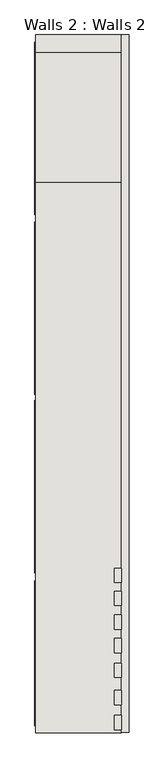
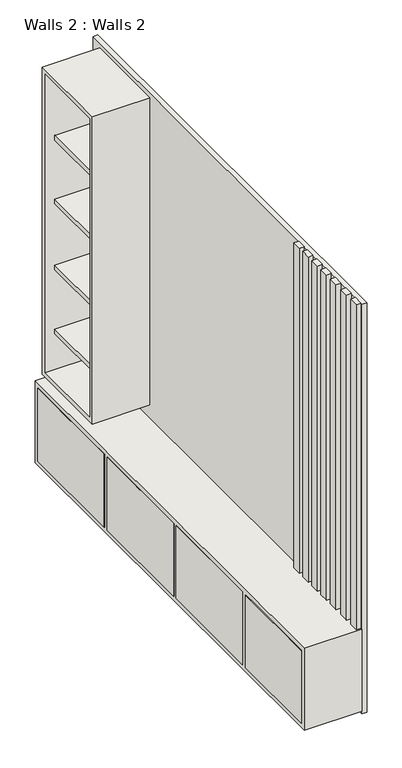
"""IFC4 building model written with IfcOpenShell, lengths in millimetres: wall geometry, Walls 2 : Walls 2."""

from ifc_helpers import new_model, si_unit, frame, origin, origin_with_axes, place, context, project, spatial, polyline, outline, extrude, faceted_brep, source, transform, mapped, element, save


def walls_2_walls_2_a3e54821(model_context):
    return source(origin(), model_context, "Body", "SolidModel", [
        extrude(outline(polyline([(-1167.1478577, -3563.611411), (-1167.1478577, -3052.3039411), (-1164.5681702, -3052.3039411), (-1164.5681702, -3563.611411), (-1167.1478577, -3563.611411)])), frame((0.0, 0.0, 40.132709), z_axis=(0.0, 0.0, 1.0), x_axis=(1.0, 0.0, 0.0)), (0.0, 0.0, 1.0), 406.4),
        extrude(outline(polyline([(-1167.1478577, -3023.861411), (-1167.1478577, -2414.261411), (-1164.5681702, -2414.261411), (-1164.5681702, -3023.861411), (-1167.1478577, -3023.861411)])), frame((0.0, 0.0, 40.132709), z_axis=(0.0, 0.0, 1.0), x_axis=(1.0, 0.0, 0.0)), (0.0, 0.0, 1.0), 406.4),
        extrude(outline(polyline([(-1167.1478577, -2393.557676), (-1167.1478577, -1783.957676), (-1164.5681702, -1783.957676), (-1164.5681702, -2393.557676), (-1167.1478577, -2393.557676)])), frame((0.0, 0.0, 40.132709), z_axis=(0.0, 0.0, 1.0), x_axis=(1.0, 0.0, 0.0)), (0.0, 0.0, 1.0), 406.4),
        extrude(outline(polyline([(-1167.1478577, -1758.557676), (-1167.1478577, -1148.957676), (-1164.5681702, -1148.957676), (-1164.5681702, -1758.557676), (-1167.1478577, -1758.557676)])), frame((0.0, 0.0, 40.132709), z_axis=(0.0, 0.0, 1.0), x_axis=(1.0, 0.0, 0.0)), (0.0, 0.0, 1.0), 406.4),
        extrude(outline(polyline([(-885.1681702, -3577.3260888), (-885.1681702, -3526.5260888), (-859.7681702, -3526.5260888), (-859.7681702, -3577.3260888), (-885.1681702, -3577.3260888)])), frame((0.0, 0.0, 471.932709), z_axis=(0.0, 0.0, 1.0), x_axis=(1.0, 0.0, 0.0)), (0.0, 0.0, 1.0), 1815.6625633),
        extrude(outline(polyline([(-885.1681702, -3489.4392633), (-885.1681702, -3438.6392633), (-859.7681702, -3438.6392633), (-859.7681702, -3489.4392633), (-885.1681702, -3489.4392633)])), frame((0.0, 0.0, 471.932709), z_axis=(0.0, 0.0, 1.0), x_axis=(1.0, 0.0, 0.0)), (0.0, 0.0, 1.0), 1815.6625633),
        extrude(outline(polyline([(-885.1681702, -3222.7392633), (-885.1681702, -3171.9392633), (-859.7681702, -3171.9392633), (-859.7681702, -3222.7392633), (-885.1681702, -3222.7392633)])), frame((0.0, 0.0, 471.932709), z_axis=(0.0, 0.0, 1.0), x_axis=(1.0, 0.0, 0.0)), (0.0, 0.0, 1.0), 1815.6625633),
        extrude(outline(polyline([(-885.1681702, -3393.1760888), (-885.1681702, -3342.3760888), (-859.7681702, -3342.3760888), (-859.7681702, -3393.1760888), (-885.1681702, -3393.1760888)])), frame((0.0, 0.0, 471.932709), z_axis=(0.0, 0.0, 1.0), x_axis=(1.0, 0.0, 0.0)), (0.0, 0.0, 1.0), 1815.6625633),
        extrude(outline(polyline([(-885.1681702, -3305.2892633), (-885.1681702, -3254.4892633), (-859.7681702, -3254.4892633), (-859.7681702, -3305.2892633), (-885.1681702, -3305.2892633)])), frame((0.0, 0.0, 471.932709), z_axis=(0.0, 0.0, 1.0), x_axis=(1.0, 0.0, 0.0)), (0.0, 0.0, 1.0), 1815.6625633),
        extrude(outline(polyline([(-885.1681702, -3139.1760888), (-885.1681702, -3088.3760888), (-859.7681702, -3088.3760888), (-859.7681702, -3139.1760888), (-885.1681702, -3139.1760888)])), frame((0.0, 0.0, 471.932709), z_axis=(0.0, 0.0, 1.0), x_axis=(1.0, 0.0, 0.0)), (0.0, 0.0, 1.0), 1815.6625633),
        extrude(outline(polyline([(-885.1681702, -3057.9595435), (-885.1681702, -3007.1595435), (-859.7681702, -3007.1595435), (-859.7681702, -3057.9595435), (-885.1681702, -3057.9595435)])), frame((0.0, 0.0, 471.932709), z_axis=(0.0, 0.0, 1.0), x_axis=(1.0, 0.0, 0.0)), (0.0, 0.0, 1.0), 1815.6625633),
        extrude(outline(polyline([(-1164.5681702, -3587.357676), (-1164.5681702, -1123.557676), (-859.7681702, -1123.557676), (-859.7681702, -3587.357676), (-1164.5681702, -3587.357676)])), frame((0.0, 0.0, 14.732709), z_axis=(0.0, 0.0, 1.0), x_axis=(1.0, 0.0, 0.0)), (0.0, 0.0, 1.0), 457.2),
        extrude(outline(polyline([(-1113.7681702, -1618.857676), (-1113.7681702, -1212.457676), (-885.1681702, -1212.457676), (-885.1681702, -1618.857676), (-1113.7681702, -1618.857676)])), frame((0.0, 0.0, 1852.4679591), z_axis=(0.0, 0.0, 1.0), x_axis=(1.0, 0.0, 0.0)), (0.0, 0.0, 1.0), 25.4),
        extrude(outline(polyline([(-1113.7681702, -1618.857676), (-1113.7681702, -1212.457676), (-885.1681702, -1212.457676), (-885.1681702, -1618.857676), (-1113.7681702, -1618.857676)])), frame((0.0, 0.0, 1496.8679591), z_axis=(0.0, 0.0, 1.0), x_axis=(1.0, 0.0, 0.0)), (0.0, 0.0, 1.0), 25.4),
        extrude(outline(polyline([(-1113.7681702, -1618.857676), (-1113.7681702, -1212.457676), (-885.1681702, -1212.457676), (-885.1681702, -1618.857676), (-1113.7681702, -1618.857676)])), frame((0.0, 0.0, 1128.5679591), z_axis=(0.0, 0.0, 1.0), x_axis=(1.0, 0.0, 0.0)), (0.0, 0.0, 1.0), 25.4),
        extrude(outline(polyline([(-1113.7681702, -1618.857676), (-1113.7681702, -1212.457676), (-885.1681702, -1212.457676), (-885.1681702, -1618.857676), (-1113.7681702, -1618.857676)])), frame((0.0, 0.0, 771.5696931), z_axis=(0.0, 0.0, 1.0), x_axis=(1.0, 0.0, 0.0)), (0.0, 0.0, 1.0), 25.4),
        faceted_brep([(-1164.5681702, -1644.257676, 2262.1952722), (-1164.5681702, -1187.057676, 2262.1952722), (-1164.5681702, -1187.057676, 545.99238), (-1164.5681702, -1644.257676, 545.99238), (-1164.5681702, -1618.857676, 2236.7952722), (-1164.5681702, -1618.857676, 571.39238), (-1164.5681702, -1212.457676, 571.39238), (-1164.5681702, -1212.457676, 2236.7952722), (-859.7681702, -1644.257676, 2262.1952722), (-859.7681702, -1644.257676, 545.99238), (-859.7681702, -1187.057676, 545.99238), (-859.7681702, -1187.057676, 2262.1952722), (-885.1681702, -1618.857676, 2236.7952722), (-885.1681702, -1212.457676, 2236.7952722), (-885.1681702, -1212.457676, 571.39238), (-885.1681702, -1618.857676, 571.39238)], [[[0, 1, 2, 3], [4, 5, 6, 7]], [[8, 9, 10, 11]], [[1, 0, 8, 11]], [[2, 1, 11, 10]], [[3, 2, 10, 9]], [[0, 3, 9, 8]], [[12, 13, 14, 15]], [[12, 15, 5, 4]], [[15, 14, 6, 5]], [[14, 13, 7, 6]], [[13, 12, 4, 7]]]),
        extrude(outline(polyline([(-859.7681702, -3587.357676), (-859.7681702, -1123.557676), (-834.3681702, -1123.557676), (-834.3681702, -3587.357676), (-859.7681702, -3587.357676)])), origin_with_axes(), (0.0, 0.0, 1.0), 2287.5952722),
    ])


if __name__ == "__main__":
    model = new_model("IFC4")
    model_context = context("Model", 3, world=origin())
    ifc_project = project(units=[si_unit("LENGTHUNIT", "METRE", prefix="MILLI")], contexts=[model_context])
    site = spatial("IfcSite", under=ifc_project)
    building = spatial("IfcBuilding", under=site)
    placement = place(None, origin())
    walls_2_walls_2_shape = walls_2_walls_2_a3e54821(model_context)
    element("IfcWall", 1, ObjectType="Walls 2 : Walls 2", at=placement, inside=building, context=model_context, shape_type="MappedRepresentation", body=[
        mapped(walls_2_walls_2_shape, transform((0.0, 0.0, 0.0), x_axis=(1.0, 0.0, 0.0), y_axis=(0.0, 1.0, 0.0), z_axis=(0.0, 0.0, 1.0))),
    ])
    save(model, "model.ifc")

# Revit data of these elements
# Element 1 (IfcWall, "Walls 2 : Walls 2")
#   Materials on its faces: "drawers", "metal", "wood"
# Materials
#   "drawers": class "Generic", colour RGB 121 66 39, transparency 0, Cost = 0
#   "metal": class "Generic", colour RGB 76 25 7, transparency 0, Cost = 0
#   "wood": class "Generic", colour RGB 255 226 181, transparency 0, Cost = 0
